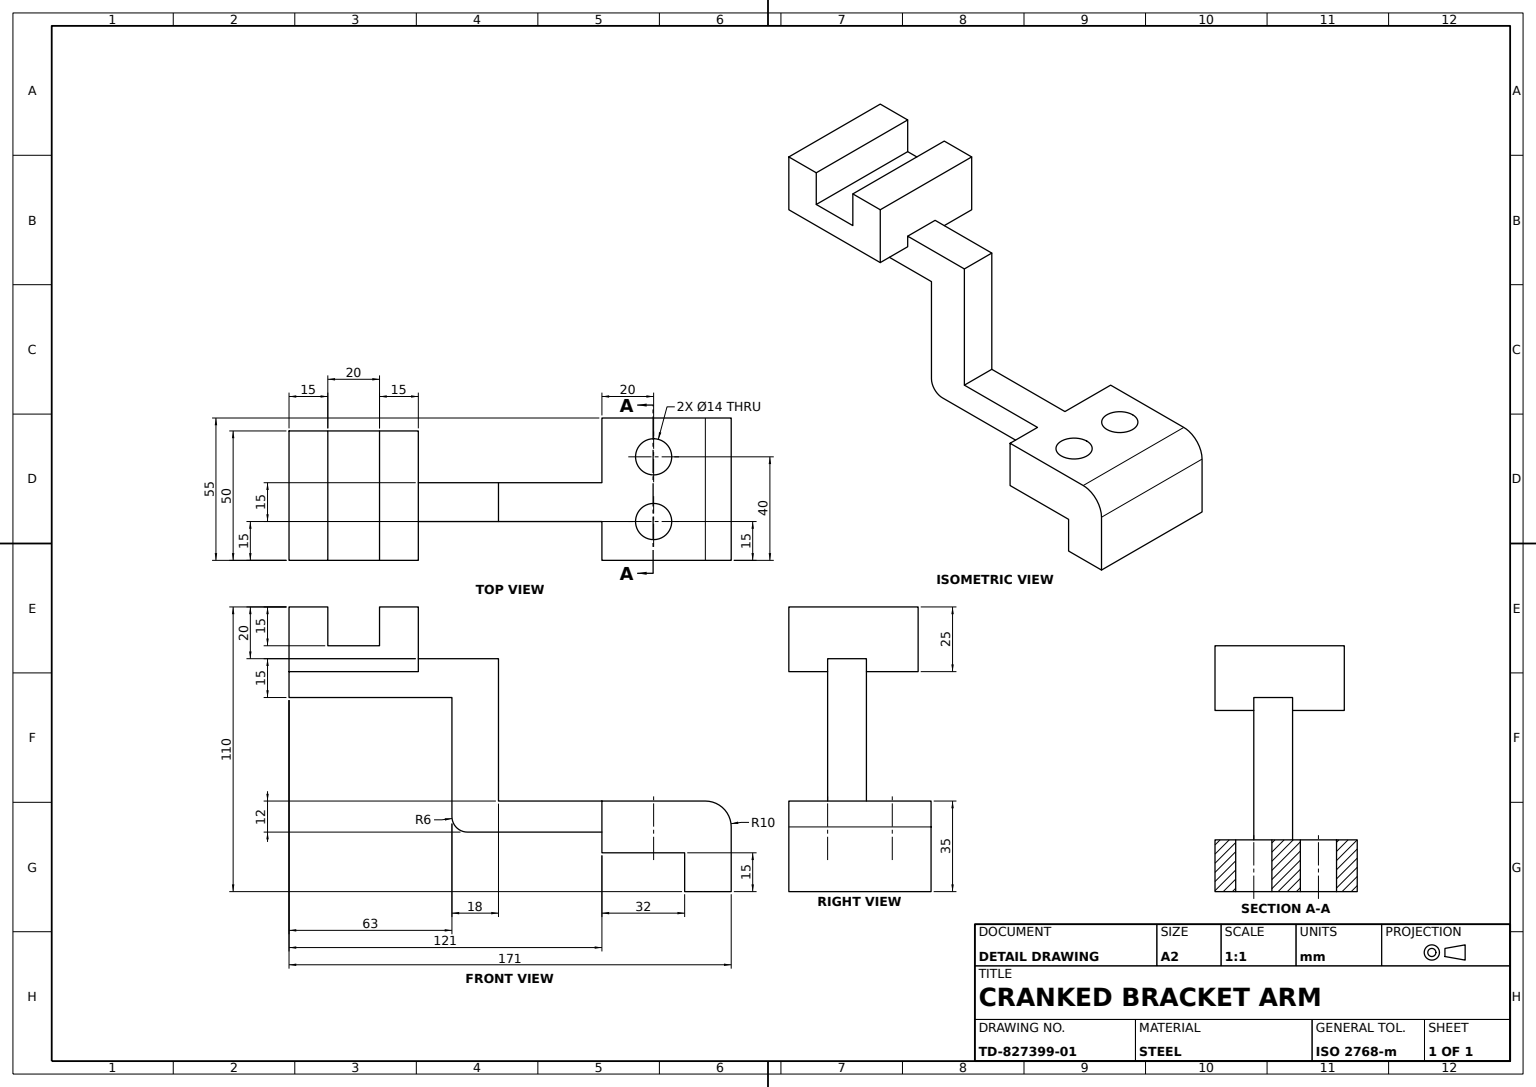
from build123d import *

# Parameters (mm, degrees)
BASE_BLOCK_DEPTH            = 55
HOLES_SKETCH_R              = 7
HOLES_2X_14_DEPTH           = 22
ARM_RISER_SKETCH_W          = 15
ARM_RISER_SKETCH_H          = 12
ARM_RISER_DEPTH             = 40
OFFSET_ARM_DEPTH            = 15
SLOTTED_CLAMP_BLOCK_DEPTH   = 35
CLAMP_BLOCK_EXTENSION_DEPTH = 15


with BuildPart() as part:
    # Base Block Profile → Base Block (new body)
    with BuildSketch(Plane.XY):
        with BuildLine():
            Line((50, -10), (50, -35))
            Line((50, -35), (32, -35))
            Line((32, -35), (32, -20))
            Line((32, -20), (0, -20))
            Line((0, -20), (0, 0))
            Line((0, 0), (40, 0))
            ThreePointArc((40, 0), (47.071067812, -2.928932188), (50, -10))
        make_face()
    extrude(amount=BASE_BLOCK_DEPTH)

    # Holes Sketch → Holes 2x_14 (cut)
    with BuildSketch(Plane(origin=(0, 0, 0), x_dir=(1, 0, 0), z_dir=(0, 1, 0))):
        with Locations(Location((20, -15, 0), (0, 0, 270))):
            Circle(HOLES_SKETCH_R)
        with Locations(Location((20, -40, 0), (0, 0, 270))):
            Circle(HOLES_SKETCH_R)
    extrude(amount=-HOLES_2X_14_DEPTH, mode=Mode.SUBTRACT)

    # Arm Riser Sketch → Arm Riser (add)
    with BuildSketch(Plane.ZY):
        with Locations((32.5, -6)):
            Rectangle(ARM_RISER_SKETCH_W, ARM_RISER_SKETCH_H)
    extrude(amount=ARM_RISER_DEPTH)

    # Offset Arm Profile → Offset Arm (add)
    with BuildSketch(Plane.XY.offset(40)):
        with BuildLine():
            Line((-40, -12), (-52, -12))
            ThreePointArc((-52, -12), (-56.242640687, -10.242640687), (-58, -6))
            Line((-58, -6), (-58, 40))
            Line((-58, 40), (-121, 40))
            Line((-121, 40), (-121, 50))
            Line((-121, 50), (-71, 50))
            Line((-71, 50), (-71, 55))
            Line((-71, 55), (-40, 55))
            Line((-40, 55), (-40, 0))
            Line((-40, 0), (0, 0))
            Line((0, 0), (0, -12))
            Line((0, -12), (-40, -12))
        make_face()
    extrude(amount=-OFFSET_ARM_DEPTH)

    # Slotted Clamp Block Profile → Slotted Clamp Block (add)
    with BuildSketch(Plane.XY.offset(40)):
        Polygon((-121, 50), (-71, 50), (-71, 75), (-86, 75), (-86, 60), (-106, 60), (-106, 75), (-121, 75), align=None)
    extrude(amount=-SLOTTED_CLAMP_BLOCK_DEPTH)

    # Clamp Block Extension Profile → Clamp Block Extension (add)
    with BuildSketch(Plane.XY.offset(40)):
        Polygon((-121, 75), (-121, 50), (-71, 50), (-71, 75), (-86, 75), (-86, 60), (-106, 60), (-106, 75), align=None)
    extrude(amount=CLAMP_BLOCK_EXTENSION_DEPTH)


solid = part.part
